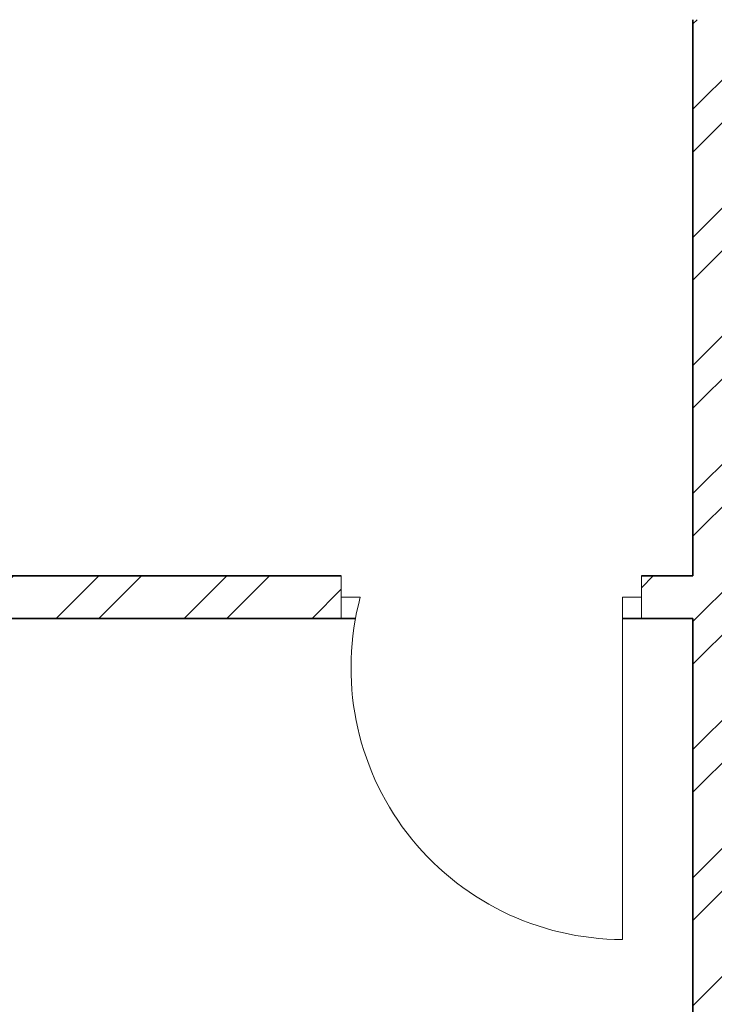
# Model space of a CAD drawing. Units: inches. Extents: x 2120 to 4013, y 1390 to 3019.
# Tile 20 of 59: x 2789 to 2862, y 1688 to 1792. Entities that reach past the tile are written whole.
import ezdxf

# ---------------------------------------------------------------- set-up
doc = ezdxf.new("R2010")
doc.units = ezdxf.units.IN
for name, color, linetype, lineweight in [('A-DOOR', 3, 'Continuous', 18), ('A-WALL', 7, 'Continuous', 35), ('A-WALL-PATT', 252, 'Continuous', 13)]:
    doc.layers.add(name, color=color, linetype=linetype, lineweight=lineweight)

# ---------------------------------------------------------------- blocks, each defined once
blk = doc.blocks.new('DOOR-SWING-36IN-105p06DEG')
for p, q in [((0, 33.75), (0, 38.25)), ((0, 38.25), (0, 36)), ((31.6, 38.25), (31.6, 33.75)), ((0, 36), (2, 36)), ((31.6, 36), (29.6, 36)), ((29.6, 36), (29.6, 0)), ((31.6, 33.75), (31.6, 36))]:
    blk.add_line(p, q)
blk.add_arc((29.6, 28.58), 28.58, 164.9445, 270)

msp = doc.modelspace()

# ---------------------------------------------------------------- hatches: boundary and pattern name
at = {"layer": 'A-WALL-PATT'}
h = msp.add_hatch(dxfattribs=at)
h.set_pattern_fill('ANSI32', color=256)
h.paths.add_polyline_path([(2271.7331, 2122.6377), (2262.7331, 2122.6377), (2262.7331, 2040.3893), (2267.2331, 2040.3893), (2271.7331, 2040.3893), (2271.7331, 2044.8856), (2271.7331, 2070.531), (2391.7331, 2070.531), (2391.7331, 1926.5306), (2388.3993, 1926.5306), (2388.3993, 1922.531), (2395.7331, 1922.531), (2395.7331, 1992.531), (2400.4511, 1992.531), (2400.4511, 1997.0306), (2395.7331, 1997.0306), (2395.7331, 2070.531), (2443.7331, 2070.531), (2443.7331, 2046.1368), (2448.2331, 2046.1368), (2448.2331, 2070.531), (2580.2331, 2070.531), (2580.2331, 1997.0306), (2492.9076, 1997.0306), (2492.9076, 1992.531), (2580.2331, 1992.531), (2580.2331, 1983.9368), (2589.2331, 1983.9368), (2589.2331, 2070.531), (2589.2331, 2075.0306), (2396.2331, 2075.0306), (2396.2331, 2184.3565), (2393.9831, 2184.3565), (2391.7331, 2184.3565), (2391.7331, 2075.0306), (2271.7331, 2075.0306)])
h.paths.add_polyline_path([(2724.7331, 2138.0306), (2628.7331, 2138.0306), (2628.7331, 2070.5306), (2628.7331, 2067.0987), (2633.2331, 2067.0987), (2637.7331, 2067.0987), (2637.7331, 2070.531), (2657.3413, 2070.531), (2657.3413, 2079.5306), (2637.7331, 2079.5306), (2637.7331, 2129.031), (2715.7331, 2129.031), (2715.7331, 2079.5306), (2698.0378, 2079.5306), (2698.0378, 2070.531), (2715.7331, 2070.531), (2715.7331, 2012.1531), (2720.2331, 2012.1531), (2724.7331, 2012.1531)])
h.paths.add_polyline_path([(2724.7331, 2213.031), (2831.3209, 2213.031), (2831.3209, 2215.281), (2831.3209, 2217.5306), (2724.7331, 2217.5306), (2724.7331, 2343.531), (2751.8755, 2343.531), (2751.8755, 2352.5306), (2715.7331, 2352.5306), (2715.7331, 2138.031), (2724.7331, 2138.031)])
h.paths.add_polyline_path([(2902.53, 2352.5306), (2811.8755, 2352.5306), (2811.8755, 2343.531), (2867.2331, 2343.531), (2867.2331, 2217.5306), (2863.6364, 2217.5306), (2863.6364, 2213.031), (2871.7331, 2213.031), (2871.7331, 2217.531), (2871.7331, 2343.531), (2902.53, 2343.531)])
h.paths.add_polyline_path([(3009.7331, 2352.5306), (2938.53, 2352.5306), (2938.53, 2343.531), (2966.2331, 2343.531), (2966.2331, 2242.3281), (2968.4831, 2242.3281), (2970.7331, 2242.3281), (2970.7331, 2343.531), (3009.7331, 2343.531)])
h.paths.add_polyline_path([(3009.7331, 2217.5306), (2970.7331, 2217.5306), (2970.7331, 2220.5422), (2968.4831, 2220.5422), (2966.2331, 2220.5422), (2966.2331, 2217.5306), (2911.7752, 2217.5306), (2907.7331, 2217.5306), (2907.7331, 2213.0306), (2907.7331, 2194.9663), (2912.2331, 2194.9663), (2912.2331, 2213.031), (2970.7331, 2213.031), (3000.7331, 2213.031), (3000.7331, 2205.523), (3009.7331, 2205.523)])
h.paths.add_polyline_path([(3009.7331, 2181.5227), (3000.7331, 2181.5227), (3000.7331, 2165.0306), (2912.2331, 2165.0306), (2912.2331, 2170.8202), (2907.7331, 2170.8202), (2907.7331, 2165.0306), (2899.5169, 2165.0306), (2899.5169, 2162.7806), (2899.5169, 2160.531), (2907.7331, 2160.531), (2907.7331, 2137.3432), (2912.2331, 2137.3432), (2912.2331, 2160.531), (3000.7331, 2160.531), (3000.7331, 2150.4993), (3009.7331, 2150.4993)])
h.paths.add_polyline_path([(3009.7331, 2126.499), (3005.2331, 2126.499), (3000.7331, 2126.499), (3000.7331, 2112.5306), (2912.2331, 2112.5306), (2912.2331, 2115.6036), (2907.7331, 2115.6036), (2907.7331, 2108.031), (3000.7331, 2108.031), (3000.7331, 2084.7256), (3009.7331, 2084.7256)], flags=17)
h.paths.add_polyline_path([(3009.7331, 1971.531), (3009.7331, 2024.7253), (3000.7331, 2024.7253), (3000.7331, 2006.4153), (3000.7331, 1971.5306), (2864.2331, 1971.5306), (2864.2331, 2160.531), (2868.0522, 2160.531), (2868.0522, 2165.0306), (2859.7331, 2165.0306), (2859.7331, 1971.5306), (2724.7331, 1971.5306), (2724.7331, 1977.7012), (2715.7331, 1977.7012), (2715.7331, 1962.5306), (2715.7331, 1950.9035), (2720.2331, 1950.9035), (2724.7331, 1950.9035), (2724.7331, 1962.531), (2855.2331, 1962.531), (2859.7331, 1962.531), (2859.7331, 1835.031), (2864.2331, 1834.8158), (2864.2331, 1962.531), (2958.7331, 1962.531), (2958.7331, 1937.0925), (2963.2331, 1937.0925), (2963.2331, 1962.531), (3000.7331, 1962.531), (3009.7331, 1962.531)])
h.paths.add_polyline_path([(2724.7331, 1728.531), (2822.7164, 1728.531), (2822.7164, 1733.0306), (2724.7331, 1733.0306), (2724.7331, 1779.3416), (2715.7331, 1779.3416), (2715.7331, 1581.531), (2753.02, 1581.531), (2753.02, 1586.031), (2753.02, 1590.5306), (2724.7331, 1590.5306)])
h.paths.add_polyline_path([(2864.2331, 1590.531), (2864.2331, 1787.031), (2868.4075, 1787.031), (2868.4075, 1791.5306), (2859.7331, 1791.5306), (2859.7331, 1739.0306), (2859.7331, 1733.0306), (2854.3125, 1733.0306), (2854.3125, 1728.531), (2859.7331, 1728.531), (2859.7331, 1590.5306), (2813.02, 1590.5306), (2813.02, 1581.531), (2868.4123, 1581.531), (2868.4123, 1583.781), (2868.4123, 1586.0306), (2864.2331, 1586.0306)])
h.paths.add_polyline_path([(3009.7331, 1754.6619), (3000.7331, 1754.6619), (3000.7331, 1739.0306), (2912.2331, 1739.0306), (2912.2331, 1742.2257), (2907.7331, 1742.2257), (2907.7331, 1739.0306), (2907.7331, 1734.531), (3000.7331, 1734.531), (3000.7331, 1590.5306), (3000.7331, 1586.0306), (2971.3921, 1586.0306), (2971.3921, 1581.531), (3009.7331, 1581.531)])
h.paths.add_polyline_path([(2911.3921, 1583.781), (2911.3921, 1586.0306), (2891.2138, 1586.0306), (2891.2138, 1581.531), (2911.3921, 1581.531)])
h.paths.add_polyline_path([(3009.7331, 1799.8422), (3000.7331, 1799.8422), (3000.7331, 1791.5306), (2912.2331, 1791.5306), (2912.2331, 1796.3264), (2909.9831, 1796.3264), (2907.7331, 1796.3264), (2907.7331, 1791.5306), (2902.7033, 1791.5306), (2902.7033, 1787.031), (2907.7331, 1787.031), (2907.7331, 1761.1622), (2912.2331, 1761.1622), (2912.2331, 1787.031), (3000.7331, 1787.031), (3000.7331, 1778.6622), (3009.7331, 1778.6622)])
h.paths.add_polyline_path([(3009.7331, 1839.5306), (2963.2331, 1839.5306), (2963.2331, 1842.8629), (2960.9831, 1842.8629), (2958.7331, 1842.8629), (2958.7331, 1839.5306), (2907.7331, 1839.5306), (2907.7331, 1814.4599), (2912.2331, 1814.4599), (2912.2331, 1835.031), (3000.7331, 1835.031), (3000.7331, 1823.8425), (3009.7331, 1823.8425), (3009.7331, 1835.031)])
h.paths.add_polyline_path([(2963.2331, 1901.0922), (2960.9831, 1901.0922), (2958.7331, 1901.0922), (2958.7331, 1862.8843), (2963.2331, 1862.8843)], flags=17)
h.paths.add_polyline_path([(2724.7331, 1891.9826), (2724.7331, 1914.3416), (2715.7331, 1914.3416), (2715.7331, 1783.8416), (2637.7331, 1783.8416), (2637.7331, 1914.3416), (2628.7331, 1914.3416), (2624.7701, 1914.3416), (2624.7701, 1909.8416), (2624.7701, 1905.3419), (2628.7331, 1905.3419), (2628.7331, 1876.9915), (2628.7331, 1779.3419), (2637.7331, 1779.3419), (2715.7331, 1779.3419), (2724.7331, 1779.3419), (2724.7331, 1835.031)])
h.paths.add_polyline_path([(2637.7331, 1731.531), (2637.7331, 1779.3416), (2628.7331, 1779.3416), (2628.7331, 1731.5306), (2589.2331, 1731.5306), (2535.9814, 1731.5306), (2496.7331, 1731.5306), (2496.7331, 1725.6876), (2498.9831, 1725.6876), (2501.2331, 1725.6876), (2501.2331, 1727.031), (2628.7331, 1727.031), (2628.7331, 1680.4203), (2628.7331, 1590.5306), (2628.7331, 1586.0306), (2604.1361, 1586.0306), (2604.1361, 1581.531), (2637.7331, 1581.531), (2637.7331, 1590.531)])

# ---------------------------------------------------------------- linework, layer by layer
at = {"layer": 'A-WALL'}
for p, q in [((2859.7331, 1739.031), (2859.7331, 1791.531)), ((2859.7331, 1739.0306), (2859.7331, 1791.5306)), ((2859.7331, 1733.031), (2859.7331, 1739.031)), ((2859.7331, 1733.0306), (2859.7331, 1739.0306)), ((2822.7164, 1733.031), (2724.7331, 1733.031)), ((2822.7164, 1733.0306), (2724.7331, 1733.0306)), ((2859.7331, 1733.031), (2854.3125, 1733.031)), ((2859.7331, 1733.0306), (2854.3125, 1733.0306)), ((2724.7331, 1728.531), (2824.2076, 1728.531)), ((2724.7331, 1728.5306), (2824.2076, 1728.5306)), ((2852.3125, 1728.531), (2859.7331, 1728.531)), ((2852.3125, 1728.5306), (2859.7331, 1728.5306)), ((2859.7331, 1590.531), (2859.7331, 1728.531)), ((2859.7331, 1590.5306), (2859.7331, 1728.5306))]:
    msp.add_line(p, q, dxfattribs=at)

# ---------------------------------------------------------------- block references
at = {"layer": 'A-DOOR'}
for p in [(2822.7164, 1694.781), (2822.7164, 1694.7806)]:
    msp.add_blockref('DOOR-SWING-36IN-105p06DEG', p, dxfattribs=at)

doc.saveas('drawing.dxf')
